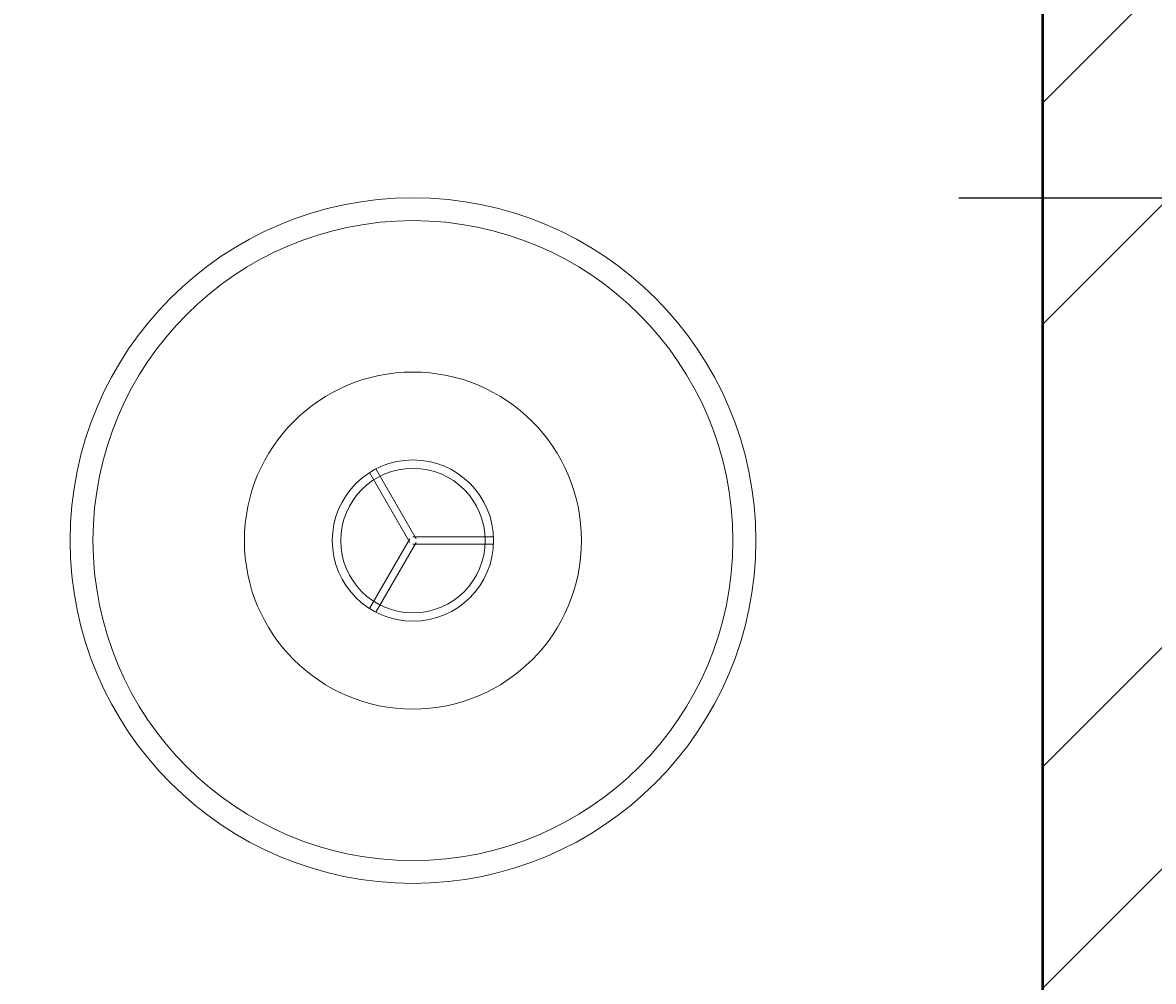
# Model space of a CAD drawing. Units: inches. Extents: x 963 to 2075, y 289 to 2657.
# Tile 26 of 98: x 1488 to 1511, y 1800 to 1820. Entities that reach past the tile are written whole.
import ezdxf

# ---------------------------------------------------------------- set-up
doc = ezdxf.new("R2010")
doc.units = ezdxf.units.IN
for name, color, linetype, lineweight in [('A-ANNO-DIMS', 2, 'Continuous', 18), ('A-FURN', 8, 'Continuous', 18), ('A-WALL', 7, 'Continuous', 50), ('A-WALL-PATT', 8, 'Continuous', 13)]:
    doc.layers.add(name, color=color, linetype=linetype, lineweight=lineweight)
doc.styles.get("Standard").update_dxf_attribs({"font": 'arial.ttf'})
doc.dimstyles.get("Standard").update_dxf_attribs({"dimtxt": 0.18, "dimasz": 0.18, "dimexe": 0.18, "dimexo": 0.0625, "dimgap": 0.09, "dimtad": 0, "dimtih": 1, "dimtoh": 1, "dimdec": 4, "dimzin": 0, "dimdsep": 46, "dimtxsty": 'Standard', "dimcen": 0.09, "dimadec": 0, "dimazin": 0, "dimtfac": 1, "dimtdec": 4, "dimtofl": 0, "dimtmove": 0, "dimatfit": 3, "dimfxl": 1, "dimtolj": 1, "dimtzin": 0, "dimarcsym": 0})

# ---------------------------------------------------------------- blocks, each defined once
blk = doc.blocks.new('SOFA-3SEAT')
at = {"ltscale": 0.03}
for p, q in [((7.593, 74.329), (6.776, 75.745)), ((7.719, 74.402), (6.902, 75.818)), ((7.593, 74.402), (6.776, 72.987)), ((7.719, 74.329), (6.902, 72.914)), ((7.656, 74.439), (9.29, 74.439)), ((7.656, 74.293), (9.29, 74.293))]:
    blk.add_line(p, q, dxfattribs=at)
for radius in [6.953, 3.418, 1.636, 1.466]:
    blk.add_circle((7.656, 74.366), radius, dxfattribs=at)
blk.add_circle((7.656, 74.366), 6.489)
blk = doc.blocks.new('*D28')
at = {"layer": 'A-ANNO-DIMS', "color": 0, "lineweight": -2, "transparency": 16777216}
for p, q in [((1506.727, 1816.319), (1519.012, 1816.319)), ((1518.832, 1816.139), (1518.832, 1775.944)), ((1518.832, 1735.382), (1518.832, 1775.577)), ((1506.727, 1735.202), (1519.012, 1735.202))]:
    blk.add_line(p, q, dxfattribs=at)
at = {"layer": 'A-ANNO-DIMS', "color": 0, "transparency": 16777216}
for points in [[(1518.802, 1816.139), (1518.862, 1816.139), (1518.832, 1816.319)], [(1518.802, 1735.382), (1518.862, 1735.382), (1518.832, 1735.202)]]:
    blk.add_solid(points, dxfattribs=at)
at = {"layer": 'Defpoints', "color": 0, "transparency": 16777216}
for p in [(1506.665, 1816.319), (1518.832, 1816.319), (1506.665, 1735.202)]:
    blk.add_point(p, dxfattribs=at)
at = {"layer": 'A-ANNO-DIMS', "color": 0, "transparency": 16777216, "insert": (1518.832, 1775.761), "char_height": 0.18, "attachment_point": 5}
blk.add_mtext('\\A1;3-SEAT SOFA 81 TYP.', dxfattribs=at)

msp = doc.modelspace()

# ---------------------------------------------------------------- hatches: boundary and pattern name
at = {"layer": 'A-WALL-PATT'}
h = msp.add_hatch(dxfattribs=at)
h.set_pattern_fill('ANSI32', color=256)
h.paths.add_polyline_path([(1473.609, 2163.068), (1473.609, 2165.318), (1376.422, 2165.318), (1376.422, 2227.983), (1371.922, 2227.983), (1371.922, 2214.818), (1368.405, 2214.818), (1368.405, 2210.318), (1371.922, 2210.318), (1371.922, 2160.818), (1395.922, 2160.818), (1395.922, 2090.318), (1217.345, 2090.318), (1217.345, 2085.818), (1395.922, 2085.818), (1458.922, 2085.818), (1458.922, 2108.318), (1454.422, 2108.318), (1454.422, 2090.318), (1400.422, 2090.318), (1400.422, 2160.818), (1473.609, 2160.818)])
h.paths.add_polyline_path([(1649.422, 2210.318), (1653.225, 2210.318), (1653.225, 2214.818), (1649.422, 2214.818), (1649.422, 2227.983), (1644.922, 2227.983), (1644.922, 2165.318), (1550.099, 2165.318), (1550.099, 2160.818), (1620.922, 2160.818), (1620.922, 2112.818), (1555.446, 2112.818), (1555.446, 2108.318), (1584.327, 2108.318), (1584.327, 2084.916), (1588.827, 2084.916), (1588.827, 2108.318), (1625.422, 2108.318), (1667.951, 2108.318), (1667.951, 2022.667), (1588.827, 2022.667), (1588.827, 2047.408), (1584.327, 2047.408), (1584.327, 1996.003), (1588.827, 1996.003), (1588.827, 2018.318), (1667.951, 2018.167), (1667.951, 1928.318), (1625.422, 1928.318), (1625.422, 1923.818), (1672.451, 1923.818), (1672.451, 1928.318), (1672.451, 1946.663), (1785.446, 1946.663), (1785.446, 1951.163), (1743.034, 1951.163), (1743.034, 2017.922), (1841.422, 2017.922), (1841.422, 2014.775), (1845.922, 2014.775), (1845.922, 2017.922), (1905.922, 2017.922), (1905.922, 1987.511), (1910.422, 1987.511), (1910.422, 2022.422), (1910.422, 2068.517), (1905.922, 2068.517), (1905.922, 2022.422), (1845.922, 2022.422), (1845.922, 2025.851), (1843.672, 2025.851), (1841.422, 2025.851), (1841.422, 2022.422), (1743.034, 2022.422), (1743.034, 2084.031), (1768.451, 2084.031), (1785.446, 2084.031), (1785.446, 2088.531), (1672.451, 2088.531), (1672.451, 2112.818), (1667.951, 2112.818), (1625.422, 2112.818), (1625.422, 2160.818), (1649.422, 2160.818)])
h.paths.add_polyline_path([(1672.451, 2084.031), (1738.534, 2084.031), (1738.534, 1951.163), (1672.451, 1951.163)], flags=16)
h.paths.add_polyline_path([(1672.451, 2084.031), (1738.534, 2084.031), (1705.492, 2017.597)], flags=0)
h.paths.add_polyline_path([(1262.766, 2085.818), (1258.266, 2085.818), (1258.266, 2023.278), (1184.422, 2023.278), (1184.422, 2018.778), (1258.266, 2018.778), (1258.266, 1950.818), (1262.766, 1950.818)])
h.paths.add_polyline_path([(1312.266, 2085.818), (1307.766, 2085.818), (1307.766, 1950.818), (1312.266, 1950.818)])
h.paths.add_polyline_path([(1458.922, 1950.818), (1395.922, 1950.818), (1216.568, 1950.818), (1216.568, 1946.318), (1346.422, 1946.318), (1395.922, 1946.318), (1395.922, 1875.818), (1371.922, 1875.818), (1371.922, 1826.318), (1368.931, 1826.318), (1368.931, 1821.818), (1371.922, 1821.818), (1371.922, 1813.622), (1376.422, 1813.622), (1376.422, 1871.318), (1474.504, 1871.318), (1474.504, 1873.568), (1474.504, 1875.818), (1400.422, 1875.818), (1400.422, 1946.318), (1454.422, 1946.318), (1454.422, 1928.318), (1458.922, 1928.318)])
h.paths.add_polyline_path([(1184.422, 2120.778), (1167.922, 2120.778), (1167.922, 2134.812), (1165.672, 2134.812), (1163.422, 2134.812), (1163.422, 2120.778), (1119.922, 2120.778), (1119.922, 2098.095), (1124.422, 2098.095), (1124.422, 2116.278), (1167.922, 2116.278), (1179.922, 2116.278), (1179.922, 2045.916), (1184.422, 2045.916), (1184.422, 2090.318), (1184.422, 2116.278)])
h.paths.add_polyline_path([(1124.422, 2018.778), (1179.922, 2018.778), (1179.922, 2016.294), (1184.422, 2016.294), (1184.422, 2023.278), (1184.422, 2026.588), (1182.172, 2026.588), (1179.922, 2026.588), (1179.922, 2023.278), (1124.422, 2023.278), (1124.422, 2074.095), (1119.922, 2074.095), (1119.922, 2018.778), (1119.922, 1979.633), (1124.422, 1979.633)])
h.paths.add_polyline_path([(1184.422, 1925.778), (1184.422, 1946.318), (1184.422, 1996.073), (1182.172, 1996.073), (1179.922, 1996.073), (1179.922, 1925.778), (1124.422, 1925.778), (1124.422, 1955.633), (1119.922, 1955.502), (1119.922, 1921.278), (1158.922, 1921.278), (1158.922, 1909.983), (1163.422, 1909.983), (1163.422, 1921.278), (1184.422, 1921.278)])
h.paths.add_polyline_path([(1341.449, 1826.318), (1163.422, 1826.318), (1163.422, 1849.983), (1158.922, 1849.983), (1158.922, 1821.818), (1158.922, 1804.033), (1163.422, 1804.033), (1163.422, 1821.818), (1341.449, 1821.818)])
h.paths.add_polyline_path([(1222.981, 1713.818), (1163.422, 1713.818), (1163.422, 1744.033), (1161.172, 1744.033), (1158.922, 1744.033), (1158.922, 1713.818), (1119.922, 1713.818), (1119.922, 1694.65), (1124.422, 1694.65), (1124.422, 1709.318), (1158.922, 1709.318), (1222.981, 1709.318)])
h.paths.add_polyline_path([(1328.422, 1713.818), (1252.042, 1713.818), (1252.042, 1711.568), (1252.042, 1709.318), (1256.422, 1709.318), (1256.422, 1547.318), (1232.937, 1547.318), (1232.937, 1545.068), (1232.937, 1542.818), (1292.422, 1542.818), (1292.422, 1527.634), (1296.922, 1527.634), (1296.922, 1542.818), (1299.464, 1542.818), (1299.464, 1547.318), (1260.922, 1547.318), (1260.922, 1658.318), (1343.661, 1658.318), (1343.661, 1660.568), (1343.661, 1662.818), (1328.422, 1662.818), (1328.422, 1676.589), (1327.402, 1676.589), (1323.922, 1676.589), (1323.922, 1662.818), (1260.922, 1662.818), (1260.922, 1709.318), (1323.922, 1709.318), (1323.922, 1699.851), (1328.422, 1699.851)])
h.paths.add_polyline_path([(1649.422, 1875.818), (1625.422, 1875.818), (1625.422, 1928.318), (1620.922, 1928.318), (1588.827, 1928.318), (1588.827, 1950.59), (1584.327, 1950.59), (1584.327, 1928.318), (1555.446, 1928.318), (1555.446, 1923.818), (1620.922, 1923.818), (1620.922, 1875.818), (1548.952, 1875.818), (1548.952, 1873.568), (1548.952, 1871.318), (1644.922, 1871.318), (1644.922, 1813.622), (1649.422, 1813.622), (1649.422, 1821.818), (1652.045, 1821.818), (1652.045, 1824.068), (1652.045, 1826.318), (1649.422, 1826.318)])
h.paths.add_polyline_path([(1512.922, 1871.318), (1516.476, 1871.318), (1516.476, 1875.818), (1512.922, 1875.818), (1512.922, 1923.818), (1512.922, 1928.318), (1512.922, 1930.827), (1508.422, 1930.827), (1508.422, 1875.818), (1504.411, 1875.818), (1504.411, 1871.318), (1508.422, 1871.318), (1508.422, 1713.818), (1376.422, 1713.818), (1376.422, 1743.325), (1371.922, 1743.325), (1371.922, 1709.318), (1371.922, 1706.01), (1376.422, 1706.01), (1376.422, 1709.318), (1508.422, 1709.318), (1508.422, 1547.318), (1501.871, 1547.318), (1501.871, 1542.818), (1508.422, 1542.818), (1508.422, 1482.818), (1508.422, 1436.318), (1512.922, 1436.318), (1512.922, 1542.818), (1519.318, 1542.818), (1519.318, 1545.068), (1519.318, 1547.318), (1512.922, 1547.318), (1512.922, 1709.318), (1644.922, 1709.318), (1644.922, 1707.548), (1649.422, 1707.548), (1649.422, 1709.318), (1649.422, 1743.325), (1644.922, 1743.325), (1644.922, 1713.818), (1512.922, 1713.818)])
h.paths.add_polyline_path([(1129.884, 1545.068), (1129.884, 1547.318), (1124.422, 1547.318), (1095.922, 1547.318), (1095.922, 1614.818), (1124.422, 1614.818), (1124.422, 1619.318), (1095.922, 1619.318), (1091.422, 1619.318), (1091.422, 1542.818), (1095.922, 1542.818), (1119.922, 1542.818), (1129.884, 1542.818)])
h.paths.add_polyline_path([(1208.422, 1542.818), (1211.74, 1542.818), (1211.74, 1547.318), (1198.851, 1547.318), (1198.851, 1542.818), (1203.922, 1542.818), (1203.922, 1478.318), (1208.422, 1478.318), (1296.922, 1478.318), (1296.922, 1503.634), (1292.422, 1503.634), (1292.422, 1482.818), (1208.422, 1482.818)])
h.paths.add_polyline_path([(1430.422, 1542.818), (1435.699, 1542.818), (1435.699, 1545.068), (1435.699, 1547.318), (1422.658, 1547.318), (1422.658, 1545.068), (1422.658, 1542.818), (1425.922, 1542.818), (1425.922, 1482.857), (1341.922, 1482.857), (1341.922, 1502.732), (1337.422, 1502.732), (1337.422, 1478.357), (1425.922, 1478.357), (1425.922, 1440.818), (1425.922, 1436.318), (1430.422, 1436.318)])
h.paths.add_polyline_path([(1698.482, 2004.259), (1727.695, 2004.259), (1727.695, 2022.916), (1698.482, 2022.916)], flags=8)

# ---------------------------------------------------------------- linework, layer by layer
at = {"layer": 'A-WALL'}
msp.add_line((1508.422, 1871.318), (1508.422, 1713.818), dxfattribs=at)

# ---------------------------------------------------------------- block references
at = {"layer": 'A-FURN'}
msp.add_blockref('SOFA-3SEAT', (1488, 1735), dxfattribs=at)

# ---------------------------------------------------------------- dimensions: what is measured, and where the dimension line sits
at = {"layer": 'A-ANNO-DIMS'}
dim = msp.add_linear_dim(base=(1518.832, 1816.319), p1=(1506.665, 1735.202), p2=(1506.665, 1816.319), angle=90, text='3-SEAT SOFA <> TYP.', dimstyle='Standard', override={"dimdec": 0, "dimlfac": 1, "dimrnd": 0, "dimzin": 0, "dimdsep": 46, "dimlunit": 2}, dxfattribs=at)
dim.commit()
dim.dimension.update_dxf_attribs({"geometry": '*D28', "text_midpoint": (1518.832, 1775.761)})

doc.saveas('drawing.dxf')
